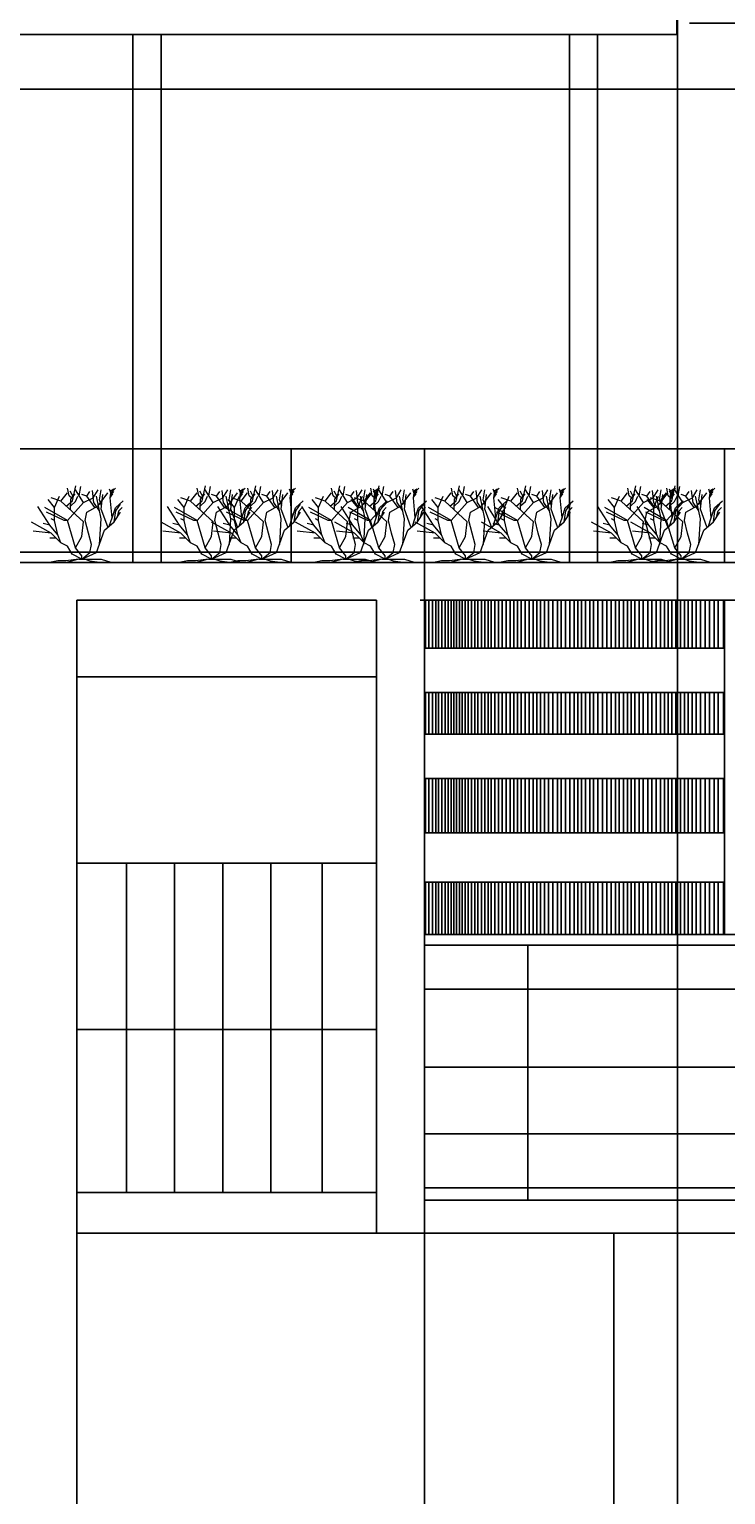
# Model space of a CAD drawing. Units: inches. Extents: x -117 to 121, y -77 to 40.
# Tile 35 of 45: x 58 to 72, y -8 to 21. Entities that reach past the tile are written whole.
import ezdxf

# ---------------------------------------------------------------- set-up
doc = ezdxf.new("R2010")
doc.units = ezdxf.units.IN
doc.header["$MEASUREMENT"] = 0
for name, color, linetype, lineweight in [('A-ANNO-DIMS', 2, 'Continuous', 18), ('A-ELEV', 7, 'Continuous', 25), ('L-PLNT', 3, 'Continuous', 13)]:
    doc.layers.add(name, color=color, linetype=linetype, lineweight=lineweight)
doc.styles.get("Standard").update_dxf_attribs({"font": 'arial.ttf'})
doc.dimstyles.get("Standard").update_dxf_attribs({"dimtxt": 0.18, "dimasz": 0.18, "dimexe": 0.18, "dimexo": 0.0625, "dimgap": 0.09, "dimtad": 0, "dimtih": 1, "dimtoh": 1, "dimdec": 4, "dimzin": 0, "dimdsep": 46, "dimtxsty": 'Standard', "dimcen": 0.09, "dimadec": 0, "dimazin": 0, "dimtfac": 1, "dimtdec": 4, "dimtofl": 0, "dimtmove": 0, "dimatfit": 3, "dimfxl": 1, "dimtolj": 1, "dimtzin": 0, "dimarcsym": 0})

# ---------------------------------------------------------------- blocks, each defined once
blk = doc.blocks.new('*U3')
for p, q in [((-12.471, 19.775), (-12.898, 22.044)), ((-11.433, 18.289), (-10.457, 22.749)), ((-9.48, 19.775), (-8.992, 22.592)), ((-0.508, 21.888), (-0.081, 20.558)), ((0.041, 20.714), (1.384, 22.044)), ((0.102, 21.34), (0.835, 21.888)), ((-16.8, 16.32), (-18.72, 18.72)), ((-14.88, 18.24), (-17.76, 19.2)), ((-16.8, 16.32), (-15.36, 19.68)), ((-14.88, 18.24), (-12.96, 20.64)), ((-8.16, 12), (-14.88, 18.24)), ((-13.325, 16.724), (-11.433, 18.289)), ((-12.96, 12.48), (-8.16, 17.76)), ((-11.677, 19.071), (-12.471, 19.775)), ((-11.28, 19.619), (-12.104, 21.184)), ((-12.043, 15.628), (-11.921, 18.836)), ((-11.982, 16.802), (-10.579, 18.054)), ((-11.921, 18.836), (-10.64, 20.401)), ((-10.579, 18.054), (-9.846, 19.697)), ((-8.16, 17.76), (-10.56, 21.6)), ((-7.2, 19.68), (-8.64, 20.16)), ((-8.16, 17.76), (-5.28, 19.2)), ((-7.2, 19.68), (-6.24, 21.12)), ((-4.8, 16.32), (-7.2, 19.68)), ((-5.086, 17.741), (-5.513, 21.34)), ((-5.28, 19.2), (-3.84, 21.6)), ((-3.377, 15.315), (-5.086, 17.819)), ((-2.88, 12.96), (-4.32, 19.68)), ((-3.84, 16.8), (-0.96, 20.64)), ((-3.377, 18.602), (-2.888, 21.575)), ((-2.766, 16.802), (-3.377, 18.602)), ((-2.88, 15.84), (-2.4, 20.16)), ((-0.203, 19.149), (0.102, 21.34)), ((0.346, 13.203), (-0.203, 19.149)), ((-0.142, 19.384), (0.59, 20.401)), ((-0.02, 20.01), (0.896, 21.105)), ((1.323, 16.254), (3.642, 18.289)), ((-18.24, 11.04), (-21.755, 16.655)), ((-12.96, 12.48), (-19.68, 16.32)), ((-13.92, 12.48), (-19.2, 14.88)), ((-16.8, 12.48), (-16.8, 16.32)), ((-7.68, 12.48), (-7.2, 14.88)), ((-7.2, 14.88), (-3.84, 16.8)), ((-0.96, 10.56), (-2.88, 15.84)), ((-0.48, 10.8), (0.346, 13.203)), ((0.346, 13.203), (1.323, 16.254)), ((0.96, 12), (1.44, 15.36)), ((0.96, 12), (2.88, 14.88)), ((1.44, 15.36), (2.88, 17.28)), ((1.92, 13.44), (2.4, 15.36)), ((2.4, 15.36), (3.36, 16.32)), ((-17.76, 8.64), (-23.663, 11.961)), ((-17.76, 8.64), (-23.128, 9.222)), ((-18.24, 11.04), (-20.16, 11.52)), ((-15.84, 8.16), (-18.24, 11.04)), ((-16.8, 12.48), (-17.76, 12.96)), ((-15.84, 8.16), (-16.8, 12.48)), ((-12.96, 12.48), (-13.92, 12.48)), ((-10.56, 4.32), (-12.96, 12.48)), ((-8.64, 7.68), (-8.16, 12)), ((-6.72, 8.64), (-7.68, 12.48)), ((-4.32, 2.88), (-1.92, 9.6)), ((-3.36, 5.28), (-2.88, 12.96)), ((-1.92, 9.6), (0.96, 12)), ((-16.32, 7.2), (-18.24, 7.2)), ((-14.88, 5.76), (-17.76, 8.64)), ((-14.88, 5.76), (-15.84, 8.16)), ((-12.96, 4.8), (-14.88, 5.76)), ((-11.52, 2.4), (-12.96, 4.8)), ((-10.56, 4.32), (-8.64, 7.68)), ((-5.76, 5.28), (-6.72, 8.64)), ((-6.24, 2.88), (-5.76, 5.28)), ((-15.84, 0.48), (-17.76, 0)), ((-13.44, 0.48), (-15.84, 0.48)), ((-9.6, 0.96), (-13.44, 0.48)), ((-9.6, 0.96), (-12.96, 0)), ((-8.64, 0.96), (-11.52, 2.4)), ((-8.64, 1.92), (-10.56, 4.32)), ((-9.6, 0.96), (-7.68, 0.96)), ((-8.64, 0.96), (-4.32, 2.88)), ((-8.64, 0.96), (-6.24, 2.88)), ((-8.64, 0.96), (-8.64, 1.92)), ((-8.64, 0.96), (-2.88, 0.96)), ((-7.68, 0.96), (-6.24, 0.48)), ((-6.24, 0.48), (-3.36, 0)), ((-2.88, 0.96), (0, 0))]:
    blk.add_line(p, q)
blk = doc.blocks.new('*D16')
at = {"layer": 'A-ANNO-DIMS', "color": 0, "lineweight": -2, "transparency": 16777216}
for p, q in [((70.862, 21.541), (120.84, 21.541)), ((120.66, 21.361), (120.66, 9.626)), ((120.66, -2.473), (120.66, 9.262)), ((87.304, -2.653), (120.84, -2.653))]:
    blk.add_line(p, q, dxfattribs=at)
at = {"layer": 'A-ANNO-DIMS', "color": 0, "transparency": 16777216}
for points in [[(120.63, 21.361), (120.69, 21.361), (120.66, 21.541)], [(120.63, -2.473), (120.69, -2.473), (120.66, -2.653)]]:
    blk.add_solid(points, dxfattribs=at)
at = {"layer": 'Defpoints', "color": 0, "transparency": 16777216}
for p in [(70.8, 21.541), (87.242, -2.653), (120.66, -2.653)]:
    blk.add_point(p, dxfattribs=at)
at = {"layer": 'A-ANNO-DIMS', "color": 0, "transparency": 16777216, "insert": (120.66, 9.444), "char_height": 0.18, "attachment_point": 5}
blk.add_mtext('\\A1;24.194', dxfattribs=at)
blk = doc.blocks.new('*D33')
at = {"layer": 'A-ANNO-DIMS', "color": 0, "lineweight": -2, "transparency": 16777216}
for p, q in [((57.433, -43.571), (57.433, 38.61)), ((57.613, 38.43), (63.572, 38.43)), ((70.441, 38.43), (64.482, 38.43)), ((70.621, -43.571), (70.621, 38.61))]:
    blk.add_line(p, q, dxfattribs=at)
at = {"layer": 'A-ANNO-DIMS', "color": 0, "transparency": 16777216}
for points in [[(57.613, 38.46), (57.613, 38.4), (57.433, 38.43)], [(70.441, 38.46), (70.441, 38.4), (70.621, 38.43)]]:
    blk.add_solid(points, dxfattribs=at)
at = {"layer": 'Defpoints', "color": 0, "transparency": 16777216}
for p in [(70.621, 38.43), (57.433, -43.633), (70.621, -43.633)]:
    blk.add_point(p, dxfattribs=at)
at = {"layer": 'A-ANNO-DIMS', "color": 0, "transparency": 16777216, "insert": (64.027, 38.43), "char_height": 0.18, "attachment_point": 5}
blk.add_mtext('\\A1;13.189', dxfattribs=at)
blk = doc.blocks.new('*D54')
at = {"layer": 'A-ANNO-DIMS', "color": 0, "lineweight": -2, "transparency": 16777216}
for p, q in [((51.654, 20.218), (120.84, 20.218)), ((120.66, 20.038), (120.66, 15.772)), ((120.66, 11.142), (120.66, 15.408)), ((51.753, 10.962), (120.84, 10.962))]:
    blk.add_line(p, q, dxfattribs=at)
at = {"layer": 'A-ANNO-DIMS', "color": 0, "transparency": 16777216}
for points in [[(120.63, 20.038), (120.69, 20.038), (120.66, 20.218)], [(120.63, 11.142), (120.69, 11.142), (120.66, 10.962)]]:
    blk.add_solid(points, dxfattribs=at)
at = {"layer": 'Defpoints', "color": 0, "transparency": 16777216}
for p in [(51.591, 20.218), (120.66, 20.218), (51.69, 10.962)]:
    blk.add_point(p, dxfattribs=at)
at = {"layer": 'A-ANNO-DIMS', "color": 0, "transparency": 16777216, "insert": (120.66, 15.59), "char_height": 0.18, "attachment_point": 5}
blk.add_mtext('\\A1;9.256', dxfattribs=at)
blk = doc.blocks.new('*D55')
at = {"layer": 'A-ANNO-DIMS', "color": 0, "lineweight": -2, "transparency": 16777216}
for p, q in [((65.473, 10.002), (120.84, 10.002)), ((120.66, 9.822), (120.66, 3.857)), ((120.66, -2.473), (120.66, 3.493)), ((65.624, -2.653), (120.84, -2.653))]:
    blk.add_line(p, q, dxfattribs=at)
at = {"layer": 'A-ANNO-DIMS', "color": 0, "transparency": 16777216}
for points in [[(120.63, 9.822), (120.69, 9.822), (120.66, 10.002)], [(120.63, -2.473), (120.69, -2.473), (120.66, -2.653)]]:
    blk.add_solid(points, dxfattribs=at)
at = {"layer": 'Defpoints', "color": 0, "transparency": 16777216}
for p in [(65.411, 10.002), (120.66, 10.002), (65.562, -2.653)]:
    blk.add_point(p, dxfattribs=at)
at = {"layer": 'A-ANNO-DIMS', "color": 0, "transparency": 16777216, "insert": (120.66, 3.675), "char_height": 0.18, "attachment_point": 5}
blk.add_mtext('\\A1;12.655', dxfattribs=at)

msp = doc.modelspace()

# ---------------------------------------------------------------- linework, layer by layer
at = {"layer": 'A-ELEV'}
for p, q in [((70.6115, 21.689), (70.6115, 21.3104)), ((32.0351, 21.3104), (70.6115, 21.3104)), ((59.7298, 21.3104), (59.7298, 10.755)), ((60.2931, 21.3104), (60.2931, 10.755)), ((68.461, 21.3104), (68.461, 10.755)), ((69.0243, 21.3104), (69.0243, 10.755)), ((70.6115, 21.3104), (70.6115, 21.3104)), ((51.6089, 13.0312), (81.0386, 13.0312)), ((62.8977, 13.0312), (62.8977, 10.755)), ((65.5651, 13.0312), (65.5651, 10.755)), ((71.5668, 13.0312), (71.5668, 10.755)), ((51.6089, 10.755), (72.955, 10.755)), ((65.5651, 10.755), (65.5651, -2.6528)), ((58.6093, 9.9998), (64.6028, 9.9998)), ((58.6093, 9.9998), (58.6093, -2.6528)), ((64.6028, 9.9998), (64.6028, -2.6528)), ((65.5651, 9.9998), (83.882, 9.9998)), ((65.5845, 9.0454), (65.5845, 9.9998)), ((65.6498, 9.0454), (65.6498, 9.9998)), ((65.7238, 9.0454), (65.7238, 9.9998)), ((65.7874, 9.0454), (65.7874, 9.9998)), ((65.845, 9.0454), (65.845, 9.9998)), ((65.9086, 9.0454), (65.9086, 9.9998)), ((65.9782, 9.0454), (65.9782, 9.9998)), ((66.0388, 9.0454), (66.0388, 9.9998)), ((66.0964, 9.0454), (66.0964, 9.9998)), ((66.1509, 9.0454), (66.1509, 9.9998)), ((66.2054, 9.0454), (66.2054, 9.9998)), ((66.2599, 9.0454), (66.2599, 9.9998)), ((66.3175, 9.0454), (66.3175, 9.9998)), ((66.375, 9.0454), (66.375, 9.9998)), ((66.436, 9.0454), (66.436, 9.9998)), ((66.5057, 9.0454), (66.5057, 9.9998)), ((66.5693, 9.0454), (66.5693, 9.9998)), ((66.6299, 9.0454), (66.6299, 9.9998)), ((66.6995, 9.0454), (66.6995, 9.9998)), ((66.7692, 9.0454), (66.7692, 9.9998)), ((66.8358, 9.0454), (66.8358, 9.9998)), ((66.8994, 9.0454), (66.8994, 9.9998)), ((66.9691, 9.0454), (66.9691, 9.9998)), ((67.0418, 9.0454), (67.0418, 9.9998)), ((67.1145, 9.0454), (67.1145, 9.9998)), ((67.1967, 9.0454), (67.1967, 9.9998)), ((67.2754, 9.0454), (67.2754, 9.9998)), ((67.3512, 9.0454), (67.3512, 9.9998)), ((67.4239, 9.0454), (67.4239, 9.9998)), ((67.4996, 9.0454), (67.4996, 9.9998)), ((67.5787, 9.0454), (67.5787, 9.9998)), ((67.6574, 9.0454), (67.6574, 9.9998)), ((67.7362, 9.0454), (67.7362, 9.9998)), ((67.8089, 9.0454), (67.8089, 9.9998)), ((67.8816, 9.0454), (67.8816, 9.9998)), ((67.9664, 9.0454), (67.9664, 9.9998)), ((68.0451, 9.0454), (68.0451, 9.9998)), ((68.1269, 9.0454), (68.1269, 9.9998)), ((68.2213, 9.0454), (68.2213, 9.9998)), ((68.3, 9.0454), (68.3, 9.9998)), ((68.3818, 9.0454), (68.3818, 9.9998)), ((68.4696, 9.0454), (68.4696, 9.9998)), ((68.5545, 9.0454), (68.5545, 9.9998)), ((68.6272, 9.0454), (68.6272, 9.9998)), ((68.7029, 9.0454), (68.7029, 9.9998)), ((68.7847, 9.0454), (68.7847, 9.9998)), ((68.8695, 9.0454), (68.8695, 9.9998)), ((68.9452, 9.0454), (68.9452, 9.9998)), ((69.0334, 9.0454), (69.0334, 9.9998)), ((69.1213, 9.0454), (69.1213, 9.9998)), ((69.2122, 9.0454), (69.2122, 9.9998)), ((69.2939, 9.0454), (69.2939, 9.9998)), ((69.3818, 9.0454), (69.3818, 9.9998)), ((69.4575, 9.0454), (69.4575, 9.9998)), ((69.5423, 9.0454), (69.5423, 9.9998)), ((69.6241, 9.0454), (69.6241, 9.9998)), ((69.6998, 9.0454), (69.6998, 9.9998)), ((69.7725, 9.0454), (69.7725, 9.9998)), ((69.8549, 9.0454), (69.8549, 9.9998)), ((69.9367, 9.0454), (69.9367, 9.9998)), ((70.0275, 9.0454), (70.0275, 9.9998)), ((70.1124, 9.0454), (70.1124, 9.9998)), ((70.1972, 9.0454), (70.1972, 9.9998)), ((70.282, 9.0454), (70.282, 9.9998)), ((70.3638, 9.0454), (70.3638, 9.9998)), ((70.4395, 9.0454), (70.4395, 9.9998)), ((70.5122, 9.0454), (70.5122, 9.9998)), ((70.594, 9.0454), (70.594, 9.9998)), ((70.6818, 9.0454), (70.6818, 9.9998)), ((70.7666, 9.0454), (70.7666, 9.9998)), ((70.8393, 9.0454), (70.8393, 9.9998)), ((70.9181, 9.0454), (70.9181, 9.9998)), ((70.9968, 9.0454), (70.9968, 9.9998)), ((71.0847, 9.0454), (71.0847, 9.9998)), ((71.1756, 9.0454), (71.1756, 9.9998)), ((71.2634, 9.0454), (71.2634, 9.9998)), ((71.3551, 9.0454), (71.3551, 9.9998)), ((71.4399, 9.0454), (71.4399, 9.9998)), ((71.5429, 9.0454), (71.5429, 9.9998)), ((71.5668, 9.9998), (71.5668, 3.3186)), ((65.5651, 9.0454), (71.5668, 9.0454)), ((58.6093, 8.4679), (64.6028, 8.4679)), ((65.5651, 8.1584), (71.5668, 8.1584)), ((65.5845, 7.3208), (65.5845, 8.1584)), ((65.6498, 7.3208), (65.6498, 8.1584)), ((65.7238, 7.3208), (65.7238, 8.1584)), ((65.7874, 7.3208), (65.7874, 8.1584)), ((65.845, 7.3208), (65.845, 8.1584)), ((65.9086, 7.3208), (65.9086, 8.1584)), ((65.9782, 7.3208), (65.9782, 8.1584)), ((66.0388, 7.3208), (66.0388, 8.1584)), ((66.0964, 7.3208), (66.0964, 8.1584)), ((66.1509, 7.3208), (66.1509, 8.1584)), ((66.2054, 7.3208), (66.2054, 8.1584)), ((66.2599, 7.3208), (66.2599, 8.1584)), ((66.3175, 7.3208), (66.3175, 8.1584)), ((66.375, 7.3208), (66.375, 8.1584)), ((66.436, 7.3208), (66.436, 8.1584)), ((66.5057, 7.3208), (66.5057, 8.1584)), ((66.5693, 7.3208), (66.5693, 8.1584)), ((66.6299, 7.3208), (66.6299, 8.1584)), ((66.6995, 7.3208), (66.6995, 8.1584)), ((66.7692, 7.3208), (66.7692, 8.1584)), ((66.8358, 7.3208), (66.8358, 8.1584)), ((66.8994, 7.3208), (66.8994, 8.1584)), ((66.9691, 7.3208), (66.9691, 8.1584)), ((67.0418, 7.3208), (67.0418, 8.1584)), ((67.1145, 7.3208), (67.1145, 8.1584)), ((67.1967, 7.3208), (67.1967, 8.1584)), ((67.2754, 7.3208), (67.2754, 8.1584)), ((67.3512, 7.3208), (67.3512, 8.1584)), ((67.4239, 7.3208), (67.4239, 8.1584)), ((67.4996, 7.3208), (67.4996, 8.1584)), ((67.5787, 7.3208), (67.5787, 8.1584)), ((67.6574, 7.3208), (67.6574, 8.1584)), ((67.7362, 7.3208), (67.7362, 8.1584)), ((67.8089, 7.3208), (67.8089, 8.1584)), ((67.8816, 7.3208), (67.8816, 8.1584)), ((67.9664, 7.3208), (67.9664, 8.1584)), ((68.0451, 7.3208), (68.0451, 8.1584)), ((68.1269, 7.3208), (68.1269, 8.1584)), ((68.2213, 7.3208), (68.2213, 8.1584)), ((68.3, 7.3208), (68.3, 8.1584)), ((68.3818, 7.3208), (68.3818, 8.1584)), ((68.4696, 7.3208), (68.4696, 8.1584)), ((68.5545, 7.3208), (68.5545, 8.1584)), ((68.6272, 7.3208), (68.6272, 8.1584)), ((68.7029, 7.3208), (68.7029, 8.1584)), ((68.7847, 7.3208), (68.7847, 8.1584)), ((68.8695, 7.3208), (68.8695, 8.1584)), ((68.9452, 7.3208), (68.9452, 8.1584)), ((69.0334, 7.3208), (69.0334, 8.1584)), ((69.1213, 7.3208), (69.1213, 8.1584)), ((69.2122, 7.3208), (69.2122, 8.1584)), ((69.2939, 7.3208), (69.2939, 8.1584)), ((69.3818, 7.3208), (69.3818, 8.1584)), ((69.4575, 7.3208), (69.4575, 8.1584)), ((69.5423, 7.3208), (69.5423, 8.1584)), ((69.6241, 7.3208), (69.6241, 8.1584)), ((69.6998, 7.3208), (69.6998, 8.1584)), ((69.7725, 7.3208), (69.7725, 8.1584)), ((69.8549, 7.3208), (69.8549, 8.1584)), ((69.9367, 7.3208), (69.9367, 8.1584)), ((70.0275, 7.3208), (70.0275, 8.1584)), ((70.1124, 7.3208), (70.1124, 8.1584)), ((70.1972, 7.3208), (70.1972, 8.1584)), ((70.282, 7.3208), (70.282, 8.1584)), ((70.3638, 7.3208), (70.3638, 8.1584)), ((70.4395, 7.3208), (70.4395, 8.1584)), ((70.5122, 7.3208), (70.5122, 8.1584)), ((70.594, 7.3208), (70.594, 8.1584)), ((70.6818, 7.3208), (70.6818, 8.1584)), ((70.7666, 7.3208), (70.7666, 8.1584)), ((70.8393, 7.3208), (70.8393, 8.1584)), ((70.9181, 7.3208), (70.9181, 8.1584)), ((70.9968, 7.3208), (70.9968, 8.1584)), ((71.0847, 7.3208), (71.0847, 8.1584)), ((71.1756, 7.3208), (71.1756, 8.1584)), ((71.2634, 7.3208), (71.2634, 8.1584)), ((71.3551, 7.3208), (71.3551, 8.1584)), ((71.4399, 7.3208), (71.4399, 8.1584)), ((71.5429, 7.3208), (71.5429, 8.1584)), ((65.5651, 7.3208), (71.5668, 7.3208)), ((65.5651, 6.4338), (71.5668, 6.4338)), ((65.5845, 5.3498), (65.5845, 6.4338)), ((65.6498, 5.3498), (65.6498, 6.4338)), ((65.7238, 5.3498), (65.7238, 6.4338)), ((65.7874, 5.3498), (65.7874, 6.4338)), ((65.845, 5.3498), (65.845, 6.4338)), ((65.9086, 5.3498), (65.9086, 6.4338)), ((65.9782, 5.3498), (65.9782, 6.4338)), ((66.0388, 5.3498), (66.0388, 6.4338)), ((66.0964, 5.3498), (66.0964, 6.4338)), ((66.1509, 5.3498), (66.1509, 6.4338)), ((66.2054, 5.3498), (66.2054, 6.4338)), ((66.2599, 5.3498), (66.2599, 6.4338)), ((66.3175, 5.3498), (66.3175, 6.4338)), ((66.375, 5.3498), (66.375, 6.4338)), ((66.436, 5.3498), (66.436, 6.4338)), ((66.5057, 5.3498), (66.5057, 6.4338)), ((66.5693, 5.3498), (66.5693, 6.4338)), ((66.6299, 5.3498), (66.6299, 6.4338)), ((66.6995, 5.3498), (66.6995, 6.4338)), ((66.7692, 5.3498), (66.7692, 6.4338)), ((66.8358, 5.3498), (66.8358, 6.4338)), ((66.8994, 5.3498), (66.8994, 6.4338)), ((66.9691, 5.3498), (66.9691, 6.4338)), ((67.0418, 5.3498), (67.0418, 6.4338)), ((67.1145, 5.3498), (67.1145, 6.4338)), ((67.1967, 5.3498), (67.1967, 6.4338)), ((67.2754, 5.3498), (67.2754, 6.4338)), ((67.3512, 5.3498), (67.3512, 6.4338)), ((67.4239, 5.3498), (67.4239, 6.4338)), ((67.4996, 5.3498), (67.4996, 6.4338)), ((67.5787, 5.3498), (67.5787, 6.4338)), ((67.6574, 5.3498), (67.6574, 6.4338)), ((67.7362, 5.3498), (67.7362, 6.4338)), ((67.8089, 5.3498), (67.8089, 6.4338)), ((67.8816, 5.3498), (67.8816, 6.4338)), ((67.9664, 5.3498), (67.9664, 6.4338)), ((68.0451, 5.3498), (68.0451, 6.4338)), ((68.1269, 5.3498), (68.1269, 6.4338)), ((68.2213, 5.3498), (68.2213, 6.4338)), ((68.3, 5.3498), (68.3, 6.4338)), ((68.3818, 5.3498), (68.3818, 6.4338)), ((68.4696, 5.3498), (68.4696, 6.4338)), ((68.5545, 5.3498), (68.5545, 6.4338)), ((68.6272, 5.3498), (68.6272, 6.4338)), ((68.7029, 5.3498), (68.7029, 6.4338)), ((68.7847, 5.3498), (68.7847, 6.4338)), ((68.8695, 5.3498), (68.8695, 6.4338)), ((68.9452, 5.3498), (68.9452, 6.4338)), ((69.0334, 5.3498), (69.0334, 6.4338)), ((69.1213, 5.3498), (69.1213, 6.4338)), ((69.2122, 5.3498), (69.2122, 6.4338)), ((69.2939, 5.3498), (69.2939, 6.4338)), ((69.3818, 5.3498), (69.3818, 6.4338)), ((69.4575, 5.3498), (69.4575, 6.4338)), ((69.5423, 5.3498), (69.5423, 6.4338)), ((69.6241, 5.3498), (69.6241, 6.4338)), ((69.6998, 5.3498), (69.6998, 6.4338)), ((69.7725, 5.3498), (69.7725, 6.4338)), ((69.8549, 5.3498), (69.8549, 6.4338)), ((69.9367, 5.3498), (69.9367, 6.4338)), ((70.0275, 5.3498), (70.0275, 6.4338)), ((70.1124, 5.3498), (70.1124, 6.4338)), ((70.1972, 5.3498), (70.1972, 6.4338)), ((70.282, 5.3498), (70.282, 6.4338)), ((70.3638, 5.3498), (70.3638, 6.4338)), ((70.4395, 5.3498), (70.4395, 6.4338)), ((70.5122, 5.3498), (70.5122, 6.4338)), ((70.594, 5.3498), (70.594, 6.4338)), ((70.6818, 5.3498), (70.6818, 6.4338)), ((70.7666, 5.3498), (70.7666, 6.4338)), ((70.8393, 5.3498), (70.8393, 6.4338)), ((70.9181, 5.3498), (70.9181, 6.4338)), ((70.9968, 5.3498), (70.9968, 6.4338)), ((71.0847, 5.3498), (71.0847, 6.4338)), ((71.1756, 5.3498), (71.1756, 6.4338)), ((71.2634, 5.3498), (71.2634, 6.4338)), ((71.3551, 5.3498), (71.3551, 6.4338)), ((71.4399, 5.3498), (71.4399, 6.4338)), ((71.5429, 5.3498), (71.5429, 6.4338)), ((65.5651, 5.3498), (71.5668, 5.3498)), ((58.6093, 4.743), (64.6028, 4.743)), ((59.5999, -1.8403), (59.5999, 4.743)), ((60.5622, -1.8403), (60.5622, 4.743)), ((61.5244, -1.8403), (61.5244, 4.743)), ((62.4867, -1.8403), (62.4867, 4.743)), ((63.5132, -1.8403), (63.5132, 4.743)), ((65.5651, 4.3643), (71.5668, 4.3643)), ((65.5845, 3.3186), (65.5845, 4.3643)), ((65.6498, 3.3186), (65.6498, 4.3643)), ((65.7238, 3.3186), (65.7238, 4.3643)), ((65.7874, 3.3186), (65.7874, 4.3643)), ((65.845, 3.3186), (65.845, 4.3643)), ((65.9086, 3.3186), (65.9086, 4.3643)), ((65.9782, 3.3186), (65.9782, 4.3643)), ((66.0388, 3.3186), (66.0388, 4.3643)), ((66.0964, 3.3186), (66.0964, 4.3643)), ((66.1509, 3.3186), (66.1509, 4.3643)), ((66.2054, 3.3186), (66.2054, 4.3643)), ((66.2599, 3.3186), (66.2599, 4.3643)), ((66.3175, 3.3186), (66.3175, 4.3643)), ((66.375, 3.3186), (66.375, 4.3643)), ((66.436, 3.3186), (66.436, 4.3643)), ((66.5057, 3.3186), (66.5057, 4.3643)), ((66.5693, 3.3186), (66.5693, 4.3643)), ((66.6299, 3.3186), (66.6299, 4.3643)), ((66.6995, 3.3186), (66.6995, 4.3643)), ((66.7692, 3.3186), (66.7692, 4.3643)), ((66.8358, 3.3186), (66.8358, 4.3643)), ((66.8994, 3.3186), (66.8994, 4.3643)), ((66.9691, 3.3186), (66.9691, 4.3643)), ((67.0418, 3.3186), (67.0418, 4.3643)), ((67.1145, 3.3186), (67.1145, 4.3643)), ((67.1967, 3.3186), (67.1967, 4.3643)), ((67.2754, 3.3186), (67.2754, 4.3643)), ((67.3512, 3.3186), (67.3512, 4.3643)), ((67.4239, 3.3186), (67.4239, 4.3643)), ((67.4996, 3.3186), (67.4996, 4.3643)), ((67.5787, 3.3186), (67.5787, 4.3643)), ((67.6574, 3.3186), (67.6574, 4.3643)), ((67.7362, 3.3186), (67.7362, 4.3643)), ((67.8089, 3.3186), (67.8089, 4.3643)), ((67.8816, 3.3186), (67.8816, 4.3643)), ((67.9664, 3.3186), (67.9664, 4.3643)), ((68.0451, 3.3186), (68.0451, 4.3643)), ((68.1269, 3.3186), (68.1269, 4.3643)), ((68.2213, 3.3186), (68.2213, 4.3643)), ((68.3, 3.3186), (68.3, 4.3643)), ((68.3818, 3.3186), (68.3818, 4.3643)), ((68.4696, 3.3186), (68.4696, 4.3643)), ((68.5545, 3.3186), (68.5545, 4.3643)), ((68.6272, 3.3186), (68.6272, 4.3643)), ((68.7029, 3.3186), (68.7029, 4.3643)), ((68.7847, 3.3186), (68.7847, 4.3643)), ((68.8695, 3.3186), (68.8695, 4.3643)), ((68.9452, 3.3186), (68.9452, 4.3643)), ((69.0334, 3.3186), (69.0334, 4.3643)), ((69.1213, 3.3186), (69.1213, 4.3643)), ((69.2122, 3.3186), (69.2122, 4.3643)), ((69.2939, 3.3186), (69.2939, 4.3643)), ((69.3818, 3.3186), (69.3818, 4.3643)), ((69.4575, 3.3186), (69.4575, 4.3643)), ((69.5423, 3.3186), (69.5423, 4.3643)), ((69.6241, 3.3186), (69.6241, 4.3643)), ((69.6998, 3.3186), (69.6998, 4.3643)), ((69.7725, 3.3186), (69.7725, 4.3643)), ((69.8549, 3.3186), (69.8549, 4.3643)), ((69.9367, 3.3186), (69.9367, 4.3643)), ((70.0275, 3.3186), (70.0275, 4.3643)), ((70.1124, 3.3186), (70.1124, 4.3643)), ((70.1972, 3.3186), (70.1972, 4.3643)), ((70.282, 3.3186), (70.282, 4.3643)), ((70.3638, 3.3186), (70.3638, 4.3643)), ((70.4395, 3.3186), (70.4395, 4.3643)), ((70.5122, 3.3186), (70.5122, 4.3643)), ((70.594, 3.3186), (70.594, 4.3643)), ((70.6818, 3.3186), (70.6818, 4.3643)), ((70.7666, 3.3186), (70.7666, 4.3643)), ((70.8393, 3.3186), (70.8393, 4.3643)), ((70.9181, 3.3186), (70.9181, 4.3643)), ((70.9968, 3.3186), (70.9968, 4.3643)), ((71.0847, 3.3186), (71.0847, 4.3643)), ((71.1756, 3.3186), (71.1756, 4.3643)), ((71.2634, 3.3186), (71.2634, 4.3643)), ((71.3551, 3.3186), (71.3551, 4.3643)), ((71.4399, 3.3186), (71.4399, 4.3643)), ((71.5429, 3.3186), (71.5429, 4.3643)), ((71.5668, 3.3186), (65.5651, 3.3186)), ((65.6498, 3.3186), (65.5651, 3.3186)), ((71.5668, 3.3186), (87.2416, 3.3186)), ((71.5668, 3.1036), (65.5651, 3.1036)), ((67.6326, -1.9953), (67.6326, 3.1036)), ((71.5668, 3.1036), (87.2416, 3.1036)), ((65.5651, 2.2251), (85.7179, 2.2251)), ((58.6093, 1.4169), (64.6028, 1.4169)), ((65.5651, 0.661), (85.7179, 0.661)), ((65.5651, -0.6675), (85.7179, -0.6675)), ((65.5651, -1.7455), (85.7179, -1.7455)), ((58.6093, -1.8403), (64.6028, -1.8403)), ((87.2416, -1.9953), (65.5651, -1.9953)), ((64.6028, -2.6528), (58.6093, -2.6528)), ((58.6093, -2.6528), (58.6093, -6.5943)), ((87.2416, -2.6528), (64.6028, -2.6528)), ((65.562, -2.6528), (65.562, -10.7374)), ((69.3498, -2.6528), (69.3498, -10.7374)), ((58.6093, -6.5943), (58.6093, -10.7374))]:
    msp.add_line(p, q, dxfattribs=at)

# ---------------------------------------------------------------- block references
at = {"layer": 'L-PLNT', "xscale": 0.0671647796176818, "yscale": 0.0671647796176818, "zscale": 0.0671647796176818}
for p in [(59.2884, 10.7596), (61.883, 10.7596), (62.891, 10.7596), (64.571, 10.7596), (65.355, 10.7596), (66.9658, 10.7596), (68.2911, 10.7596), (70.4937, 10.7596), (71.2777, 10.7596)]:
    msp.add_blockref('*U3', p, dxfattribs=at)

# ---------------------------------------------------------------- dimensions: what is measured, and where the dimension line sits
at = {"layer": 'A-ANNO-DIMS'}
dim = msp.add_linear_dim(base=(70.6214, 38.4297), p1=(57.4328, -43.6334), p2=(70.6214, -43.6334), dimstyle='Standard', override={"dimdec": 3, "dimlfac": 1, "dimrnd": 0, "dimzin": 0, "dimdsep": 46, "dimlunit": 2}, dxfattribs=at)
dim.commit()
dim.dimension.update_dxf_attribs({"geometry": '*D33', "text_midpoint": (64.0271, 38.4297)})
for base, p1, p2, picture, middle in [((120.6602, -2.6528), (70.8, 21.5414), (87.2416, -2.6528), '*D16', (120.6602, 9.4443)), ((120.6602, 20.2181), (51.6901, 10.9623), (51.5915, 20.2181), '*D54', (120.6602, 15.5902)), ((120.6602, 10.0025), (65.562, -2.6528), (65.4109, 10.0025), '*D55', (120.6602, 3.6749))]:
    dim = msp.add_linear_dim(base=base, p1=p1, p2=p2, angle=90, dimstyle='Standard', override={"dimdec": 3, "dimlfac": 1, "dimrnd": 0, "dimzin": 0, "dimdsep": 46, "dimlunit": 2}, dxfattribs=at)
    dim.commit()
    dim.dimension.update_dxf_attribs({"geometry": picture, "text_midpoint": middle})

doc.saveas('drawing.dxf')
